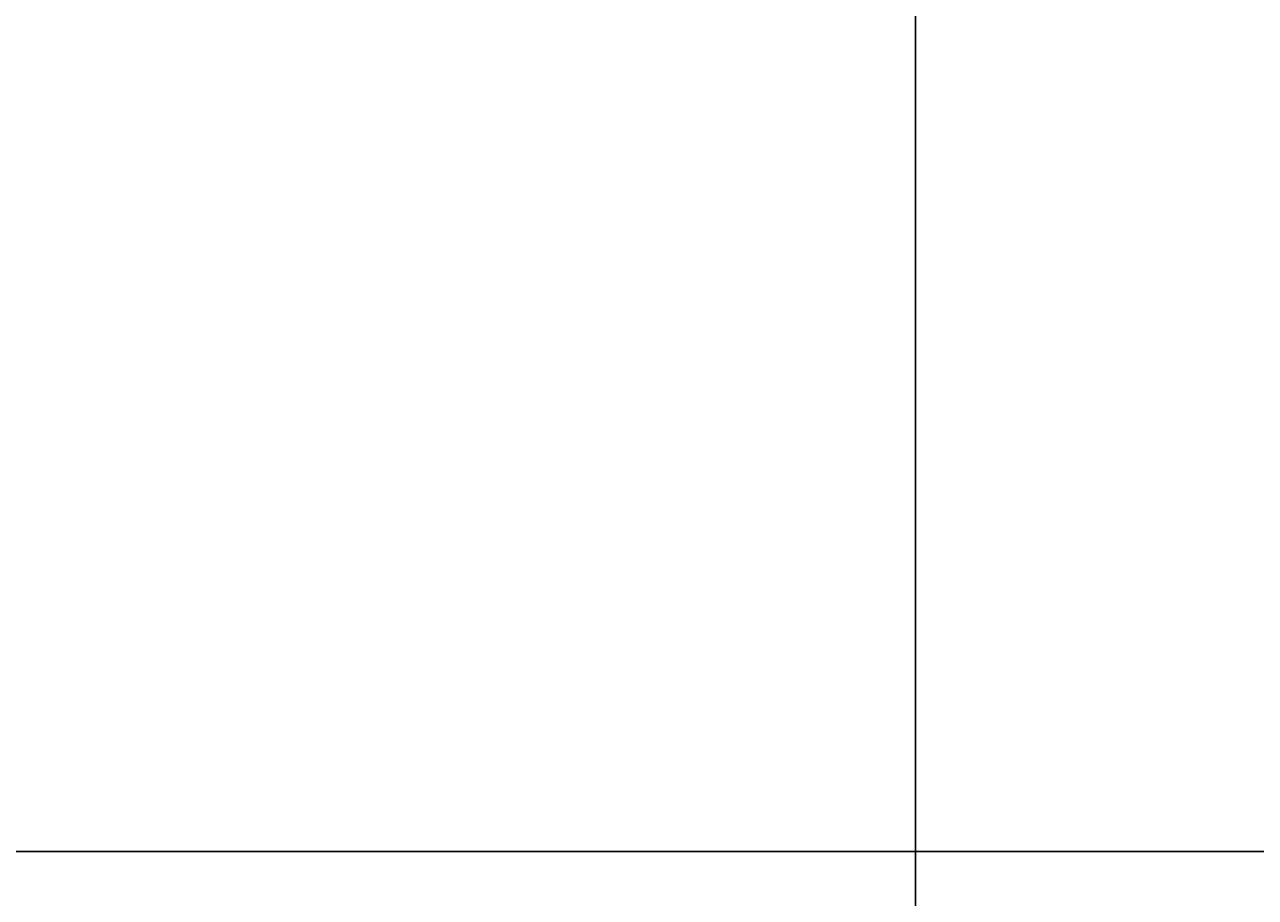
# Model space of a CAD drawing. Units: inches. Extents: x 35362 to 73946, y 43607 to 67532.
# Tile 112 of 134: x 50977 to 51049, y 48917 to 48969. Entities that reach past the tile are written whole.
import ezdxf

# ---------------------------------------------------------------- set-up
doc = ezdxf.new("R2010")
doc.units = ezdxf.units.IN
doc.header["$MEASUREMENT"] = 0
doc.layers.add('A-ANNO-DIMS', color=2, linetype='Continuous', lineweight=18)
doc.styles.get("Standard").update_dxf_attribs({"font": 'arial.ttf'})
doc.dimstyles.get("Standard").update_dxf_attribs({"dimtxt": 0.18, "dimasz": 0.18, "dimexe": 0.18, "dimexo": 0.0625, "dimgap": 0.09, "dimtad": 0, "dimtih": 1, "dimtoh": 1, "dimdec": 4, "dimzin": 0, "dimdsep": 46, "dimtxsty": 'Standard', "dimcen": 0.09, "dimadec": 0, "dimazin": 0, "dimtfac": 1, "dimtdec": 4, "dimtofl": 0, "dimtmove": 0, "dimatfit": 3, "dimfxl": 1, "dimtolj": 1, "dimtzin": 0, "dimarcsym": 0})

# ---------------------------------------------------------------- blocks, each defined once
blk = doc.blocks.new('*D11')
at = {"layer": 'A-ANNO-DIMS', "color": 0, "lineweight": -2, "transparency": 16777216}
for p, q in [((47978.665, 56028.774), (47978.665, 43606.679)), ((53109.76, 56028.774), (53109.76, 43606.679)), ((47978.845, 43606.859), (50543.871, 43606.859)), ((53109.58, 43606.859), (50544.554, 43606.859))]:
    blk.add_line(p, q, dxfattribs=at)
at = {"layer": 'A-ANNO-DIMS', "color": 0, "transparency": 16777216}
for points in [[(47978.845, 43606.889), (47978.845, 43606.829), (47978.665, 43606.859)], [(53109.58, 43606.889), (53109.58, 43606.829), (53109.76, 43606.859)]]:
    blk.add_solid(points, dxfattribs=at)
at = {"layer": 'Defpoints', "color": 0, "transparency": 16777216}
for p in [(47978.665, 56028.836), (53109.76, 56028.836), (53109.76, 43606.859)]:
    blk.add_point(p, dxfattribs=at)
at = {"layer": 'A-ANNO-DIMS', "color": 0, "transparency": 16777216, "insert": (50544.212, 43606.859), "char_height": 0.18, "attachment_point": 5}
blk.add_mtext('\\A1;5131', dxfattribs=at)
blk = doc.blocks.new('*D13')
at = {"layer": 'A-ANNO-DIMS', "color": 0, "lineweight": -2, "transparency": 16777216}
for p, q in [((48373.492, 51694.025), (48373.492, 43606.679)), ((51029.043, 51694.025), (51029.043, 43606.679)), ((48373.672, 43606.859), (49700.802, 43606.859)), ((51028.863, 43606.859), (49701.733, 43606.859))]:
    blk.add_line(p, q, dxfattribs=at)
at = {"layer": 'A-ANNO-DIMS', "color": 0, "transparency": 16777216}
for points in [[(48373.672, 43606.889), (48373.672, 43606.829), (48373.492, 43606.859)], [(51028.863, 43606.889), (51028.863, 43606.829), (51029.043, 43606.859)]]:
    blk.add_solid(points, dxfattribs=at)
at = {"layer": 'Defpoints', "color": 0, "transparency": 16777216}
for p in [(48373.492, 51694.087), (51029.043, 51694.087), (51029.043, 43606.859)]:
    blk.add_point(p, dxfattribs=at)
at = {"layer": 'A-ANNO-DIMS', "color": 0, "transparency": 16777216, "insert": (49701.267, 43606.859), "char_height": 0.18, "attachment_point": 5}
blk.add_mtext('\\A1;2655.6', dxfattribs=at)
blk = doc.blocks.new('*D17')
at = {"layer": 'A-ANNO-DIMS', "color": 0, "lineweight": -2, "transparency": 16777216}
for p, q in [((49923.307, 61293.224), (49923.307, 43606.679)), ((51913.931, 61293.224), (51913.931, 43606.679)), ((49923.487, 43606.859), (50918.164, 43606.859)), ((51913.751, 43606.859), (50919.074, 43606.859))]:
    blk.add_line(p, q, dxfattribs=at)
at = {"layer": 'A-ANNO-DIMS', "color": 0, "transparency": 16777216}
for points in [[(49923.487, 43606.889), (49923.487, 43606.829), (49923.307, 43606.859)], [(51913.751, 43606.889), (51913.751, 43606.829), (51913.931, 43606.859)]]:
    blk.add_solid(points, dxfattribs=at)
at = {"layer": 'Defpoints', "color": 0, "transparency": 16777216}
for p in [(49923.307, 61293.286), (51913.931, 61293.286), (51913.931, 43606.859)]:
    blk.add_point(p, dxfattribs=at)
at = {"layer": 'A-ANNO-DIMS', "color": 0, "transparency": 16777216, "insert": (50918.619, 43606.859), "char_height": 0.18, "attachment_point": 5}
blk.add_mtext('\\A1;1990.6', dxfattribs=at)
blk = doc.blocks.new('*D67')
at = {"layer": 'A-ANNO-DIMS', "color": 0, "lineweight": -2, "transparency": 16777216}
for p, q in [((56873.539, 53351.529), (35361.769, 53351.529)), ((35361.949, 53351.349), (35361.949, 49400.893)), ((35361.949, 45450.074), (35361.949, 49400.53)), ((53793.575, 45449.894), (35361.769, 45449.894))]:
    blk.add_line(p, q, dxfattribs=at)
at = {"layer": 'A-ANNO-DIMS', "color": 0, "transparency": 16777216}
for points in [[(35361.919, 53351.349), (35361.979, 53351.349), (35361.949, 53351.529)], [(35361.919, 45450.074), (35361.979, 45450.074), (35361.949, 45449.894)]]:
    blk.add_solid(points, dxfattribs=at)
at = {"layer": 'Defpoints', "color": 0, "transparency": 16777216}
for p in [(35361.949, 53351.529), (56873.602, 53351.529), (53793.638, 45449.894)]:
    blk.add_point(p, dxfattribs=at)
at = {"layer": 'A-ANNO-DIMS', "color": 0, "transparency": 16777216, "insert": (35361.949, 49400.712), "char_height": 0.18, "attachment_point": 5}
blk.add_mtext('\\A1;7901.6', dxfattribs=at)
blk = doc.blocks.new('*D86')
at = {"layer": 'A-ANNO-DIMS', "color": 0, "lineweight": -2, "transparency": 16777216}
for p, q in [((51285.532, 49320.079), (35361.769, 49320.079)), ((35361.949, 49319.899), (35361.949, 49120.261)), ((35361.949, 48920.259), (35361.949, 49119.897)), ((51285.532, 48920.079), (35361.769, 48920.079))]:
    blk.add_line(p, q, dxfattribs=at)
at = {"layer": 'A-ANNO-DIMS', "color": 0, "transparency": 16777216}
for points in [[(35361.919, 49319.899), (35361.979, 49319.899), (35361.949, 49320.079)], [(35361.919, 48920.259), (35361.979, 48920.259), (35361.949, 48920.079)]]:
    blk.add_solid(points, dxfattribs=at)
at = {"layer": 'Defpoints', "color": 0, "transparency": 16777216}
for p in [(35361.949, 49320.079), (51285.595, 49320.079), (51285.595, 48920.079)]:
    blk.add_point(p, dxfattribs=at)
at = {"layer": 'A-ANNO-DIMS', "color": 0, "transparency": 16777216, "insert": (35361.949, 49120.079), "char_height": 0.18, "attachment_point": 5}
blk.add_mtext('\\A1;400.0', dxfattribs=at)
blk = doc.blocks.new('*D107')
at = {"layer": 'A-ANNO-DIMS', "color": 0, "lineweight": -2, "transparency": 16777216}
for p, q in [((50139.563, 59850.014), (50139.563, 43606.679)), ((51320.813, 59850.014), (51320.813, 43606.679)), ((50139.743, 43606.859), (50729.733, 43606.859)), ((51320.633, 43606.859), (50730.643, 43606.859))]:
    blk.add_line(p, q, dxfattribs=at)
at = {"layer": 'A-ANNO-DIMS', "color": 0, "transparency": 16777216}
for points in [[(50139.743, 43606.889), (50139.743, 43606.829), (50139.563, 43606.859)], [(51320.633, 43606.889), (51320.633, 43606.829), (51320.813, 43606.859)]]:
    blk.add_solid(points, dxfattribs=at)
at = {"layer": 'Defpoints', "color": 0, "transparency": 16777216}
for p in [(50139.563, 59850.077), (51320.813, 59850.077), (51320.813, 43606.859)]:
    blk.add_point(p, dxfattribs=at)
at = {"layer": 'A-ANNO-DIMS', "color": 0, "transparency": 16777216, "insert": (50730.188, 43606.859), "char_height": 0.18, "attachment_point": 5}
blk.add_mtext('\\A1;1181.3', dxfattribs=at)

msp = doc.modelspace()

# ---------------------------------------------------------------- dimensions: what is measured, and where the dimension line sits
at = {"layer": 'A-ANNO-DIMS'}
for base, p1, p2, override, picture, middle in [((51913.931, 43606.859), (49923.307, 61293.286), (51913.931, 61293.286), {"dimdec": 1, "dimlfac": 1, "dimrnd": 0, "dimzin": 0, "dimdsep": 46, "dimlunit": 2}, '*D17', (50918.619, 43606.859)), ((51320.8133, 43606.859), (50139.5627, 59850.0769), (51320.8133, 59850.0769), {"dimdec": 1, "dimlfac": 1, "dimrnd": 0, "dimzin": 0, "dimdsep": 46, "dimlunit": 2}, '*D107', (50730.188, 43606.859)), ((53109.76, 43606.859), (47978.665, 56028.836), (53109.76, 56028.836), {"dimdec": 0, "dimlfac": 1, "dimrnd": 0, "dimzin": 0, "dimdsep": 46, "dimlunit": 2}, '*D11', (50544.212, 43606.859)), ((51029.043, 43606.859), (48373.492, 51694.087), (51029.043, 51694.087), {"dimdec": 1, "dimlfac": 1, "dimrnd": 0, "dimzin": 0, "dimdsep": 46, "dimlunit": 2}, '*D13', (49701.267, 43606.859))]:
    dim = msp.add_linear_dim(base=base, p1=p1, p2=p2, dimstyle='Standard', override=override, dxfattribs=at)
    dim.commit()
    dim.dimension.update_dxf_attribs({"geometry": picture, "text_midpoint": middle})
for base, p1, p2, picture, middle in [((35361.949, 53351.529), (53793.638, 45449.894), (56873.602, 53351.529), '*D67', (35361.949, 49400.712)), ((35361.949, 49320.079), (51285.595, 48920.079), (51285.595, 49320.079), '*D86', (35361.949, 49120.079))]:
    dim = msp.add_linear_dim(base=base, p1=p1, p2=p2, angle=90, dimstyle='Standard', override={"dimdec": 1, "dimlfac": 1, "dimrnd": 0, "dimzin": 0, "dimdsep": 46, "dimlunit": 2}, dxfattribs=at)
    dim.commit()
    dim.dimension.update_dxf_attribs({"geometry": picture, "text_midpoint": middle})

doc.saveas('drawing.dxf')
